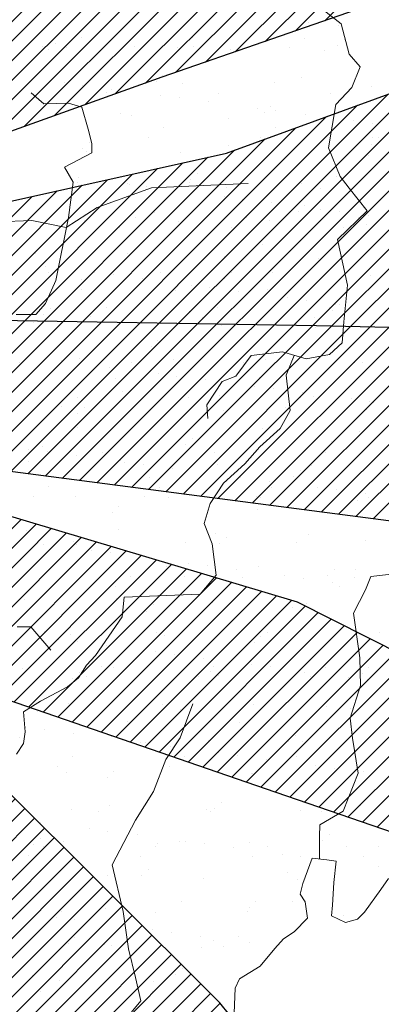
# Model space of a CAD drawing. Units: inches. Extents: x 1986 to 21484, y -1816 to 2016.
# Tile 30 of 85: x 2179.1 to 2183.13, y 1876.39 to 1887.36. Entities that reach past the tile are written whole.
import ezdxf

# ---------------------------------------------------------------- set-up
doc = ezdxf.new("R2010")
doc.units = ezdxf.units.IN
doc.layers.add('L-PLNT', color=84, linetype='Continuous', lineweight=13)
doc.layers.add('vfolhas', color=114, linetype='Continuous', lineweight=5)
for name, color, linetype in [('vfolha', 72, 'Continuous'), ('vfolha2', 110, 'Continuous'), ('vfolhas2', 102, 'Continuous')]:
    doc.layers.add(name, color=color, linetype=linetype)
pattern_1 = [(45, (-2446.5133113, 50.986076), (-0.004419417382, 0.004419417382), [])]

# ---------------------------------------------------------------- blocks, each defined once
blk = doc.blocks.new('arbusto_PB_verde_grande')
at = {"layer": 'vfolha2'}
h = blk.add_hatch(dxfattribs=at)
h.set_pattern_fill('ANSI31', color=256, scale=0.05, style=0)
h.set_pattern_definition(pattern_1)
h.paths.add_polyline_path([(0.02944, 0.35651), (0.00028, 0.09048), (0.02625, -0.03934), (0.047, 0.06233), (0.06189, 0.09731), (0.09372, 0.26573), (0.09955, 0.43473), (0.08789, 0.61313), (0.0645, 0.72266), (0.04988, 0.6851), (0.0236, 0.51294)])
h.paths.add_polyline_path([(0.30106, 0.43789), (0.14225, 0.24871), (0.26685, 0.30022)])
h.paths.add_polyline_path([(0.37995, 0.22817), (0.23697, 0.15193), (0.18428, 0.09364), (0.11122, 0.04358), (0.02625, -0.03934), (0.28061, 0.04667), (0.36829, 0.07798), (0.46756, 0.11239), (0.61068, 0.19376), (0.71585, 0.27823), (0.55813, 0.25948)])
h.paths.add_polyline_path([(0.56101, -0.29441), (0.72752, -0.32573), (0.59024, -0.2412), (0.42962, -0.15982), (0.02625, -0.03934), (0.14922, -0.14107), (0.18838, -0.16604), (0.41501, -0.24435)])
h.paths.add_polyline_path([(-0.27429, -0.44776), (-0.30352, -0.72628), (-0.23923, -0.64175), (-0.15457, -0.45716), (0.02625, -0.03934), (-0.16328, -0.25376)])
h.paths.add_polyline_path([(-0.51963, -0.24744), (-0.67736, -0.32573), (-0.59558, -0.35072), (-0.40574, -0.32882), (-0.21007, -0.20995), (0.02625, -0.03934), (-0.14874, -0.06595), (-0.31518, -0.09101), (-0.41452, -0.15048)])
h.paths.add_polyline_path([(-0.52546, 0.25007), (-0.70947, 0.24698), (-0.51963, 0.1093), (-0.32979, 0.02167), (-0.07567, -0.0128), (-0.04234, -0.02148), (-0.35024, 0.1312)])
at = {"layer": 'vfolhas'}
h = blk.add_hatch(dxfattribs=at)
h.set_pattern_fill('ANSI31', color=256, scale=0.05, style=0)
h.set_pattern_definition(pattern_1)
h.paths.add_polyline_path([(-0.07279, 0.50669), (-0.18085, 0.65063), (-0.2334, 0.67253), (-0.20712, 0.53176), (-0.10785, 0.25007), (0.02625, -0.03934), (0.00028, 0.09048), (0.00816, 0.16241), (-0.04939, 0.29079)])
h.paths.add_polyline_path([(0.09902, 0.41929), (0.09372, 0.26573), (0.07906, 0.18814), (0.15506, 0.36901), (0.26606, 0.5505), (0.28356, 0.63504), (0.2485, 0.68819), (0.25145, 0.63504), (0.20178, 0.54426)])
h.paths.add_polyline_path([(0.12295, 0.24073), (0.047, 0.06233), (0.02625, -0.03934), (0.11122, 0.04358), (0.18428, 0.09364), (0.27478, 0.19376), (0.3215, 0.25323), (0.44129, 0.38467), (0.47634, 0.57866), (0.41789, 0.45347), (0.28939, 0.30954)])
h.paths.add_polyline_path([(0.58145, -0.03779), (0.70707, 0.01536), (0.78591, 0.04667), (0.74796, 0.06549), (0.62818, 0.08423), (0.52595, 0.09048), (0.39745, 0.04358), (0.02625, -0.03934), (0.25728, -0.03154), (0.43834, -0.0347)])
h.paths.add_polyline_path([(0.52022, -0.03647), (0.43834, -0.0347), (0.25728, -0.03154), (0.02625, -0.03934), (0.17964, -0.08515), (0.53768, -0.13167), (0.69541, -0.15357), (0.78591, -0.07852), (0.70413, -0.10042)])
h.paths.add_polyline_path([(0.27189, -0.21929), (0.14922, -0.14107), (0.02625, -0.03934), (0.15794, -0.31007), (0.29522, -0.42585), (0.41789, -0.49157), (0.56396, -0.56669), (0.5114, -0.48532), (0.39456, -0.34139)])
h.paths.add_polyline_path([(-0.05818, -0.47591), (-0.02312, -0.61984), (0.047, -0.80134), (0.08494, -0.59794), (0.07911, -0.4071), (0.03527, -0.25376), (0.02625, -0.03934), (-0.03773, -0.26001)])
h.paths.add_polyline_path([(-0.24218, 0.14054), (-0.11073, 0.06858), (0.02625, -0.03934), (-0.04235, 0.10871), (-0.21007, 0.23757), (-0.36485, 0.33145), (-0.47874, 0.40341), (-0.54303, 0.46288), (-0.49041, 0.33145), (-0.39408, 0.22192)])
at = {"layer": 'vfolha'}
for p, q in [((0.53768, -0.13167), (0.17964, -0.08515)), ((0.39456, -0.34139), (0.27189, -0.21929)), ((0.5114, -0.48532), (0.39456, -0.34139))]:
    blk.add_line(p, q, dxfattribs=at)
at = {"layer": 'vfolha2'}
for p, q in [((0.36829, 0.07798), (0.28061, 0.04667)), ((0.42962, -0.15982), (0.02625, -0.03934)), ((0.59024, -0.2412), (0.42962, -0.15982)), ((0.18838, -0.16604), (0.41501, -0.24435)), ((0.41501, -0.24435), (0.56101, -0.29441))]:
    blk.add_line(p, q, dxfattribs=at)
at = {"layer": 'vfolhas2'}
for p, q in [((0.46756, 0.11239), (0.36829, 0.07798)), ((0.39745, 0.04358), (0.52595, 0.09048)), ((0.02625, -0.03934), (0.39745, 0.04358)), ((0.43834, -0.0347), (0.25728, -0.03154)), ((0.58145, -0.03779), (0.43834, -0.0347))]:
    blk.add_line(p, q, dxfattribs=at)
blk = doc.blocks.new('PLANT-SHRUB')
for p, q in [((2182.269, 1887.643), (2182.682, 1887.317)), ((2182.322, 1887.338), (2182.322, 1887.338)), ((2182.647, 1887.295), (2182.647, 1887.295)), ((2182.682, 1887.317), (2182.772, 1886.981)), ((2182.682, 1887.317), (2182.682, 1887.317)), ((2179.784, 1887.163), (2179.784, 1887.163)), ((2181.029, 1887.161), (2181.029, 1887.161)), ((2182.274, 1887.159), (2182.274, 1887.159)), ((2179.352, 1887.066), (2179.352, 1887.066)), ((2179.492, 1887.099), (2179.492, 1887.099)), ((2179.616, 1887.056), (2179.616, 1887.056)), ((2180.374, 1887.071), (2180.374, 1887.071)), ((2180.861, 1887.054), (2180.861, 1887.054)), ((2181.041, 1887.066), (2181.041, 1887.066)), ((2182.105, 1887.051), (2182.105, 1887.051)), ((2182.641, 1887.08), (2182.641, 1887.08)), ((2182.714, 1887.148), (2182.714, 1887.148)), ((2179.419, 1887.031), (2179.419, 1887.031)), ((2181.453, 1887.032), (2181.453, 1887.032)), ((2182.5, 1887.018), (2182.5, 1887.018)), ((2182.772, 1886.981), (2182.892, 1886.841)), ((2182.892, 1886.841), (2182.802, 1886.61)), ((2182.892, 1886.841), (2182.892, 1886.841)), ((2180.694, 1886.748), (2180.694, 1886.748)), ((2182.243, 1886.716), (2182.243, 1886.716)), ((2179.594, 1886.662), (2179.594, 1886.662)), ((2179.802, 1886.635), (2179.802, 1886.635)), ((2179.867, 1886.67), (2179.867, 1886.67)), ((2180.62, 1886.68), (2180.62, 1886.68)), ((2180.913, 1886.657), (2180.913, 1886.657)), ((2181.935, 1886.662), (2181.935, 1886.662)), ((2182.802, 1886.61), (2182.621, 1886.419)), ((2183.015, 1886.623), (2183.015, 1886.623)), ((2179.227, 1886.548), (2179.368, 1886.425)), ((2180.068, 1886.549), (2180.068, 1886.549)), ((2180.127, 1886.592), (2180.127, 1886.592)), ((2180.67, 1886.52), (2180.67, 1886.52)), ((2180.878, 1886.493), (2180.878, 1886.493)), ((2181.313, 1886.547), (2181.313, 1886.547)), ((2182.558, 1886.544), (2182.558, 1886.544)), ((2179.368, 1886.425), (2179.641, 1886.434)), ((2179.641, 1886.434), (2179.79, 1886.39)), ((2179.79, 1886.39), (2179.86, 1886.144)), ((2181.203, 1886.45), (2181.203, 1886.45)), ((2181.895, 1886.397), (2181.895, 1886.397)), ((2182.621, 1886.419), (2182.54, 1885.937)), ((2180.222, 1886.316), (2180.222, 1886.316)), ((2180.349, 1886.301), (2180.349, 1886.301)), ((2181.746, 1886.379), (2181.746, 1886.379)), ((2181.822, 1886.329), (2181.822, 1886.329)), ((2181.954, 1886.351), (2181.954, 1886.351)), ((2182.279, 1886.309), (2182.279, 1886.309)), ((2181.428, 1886.262), (2181.428, 1886.262)), ((2182.474, 1886.248), (2182.474, 1886.248)), ((2182.822, 1886.237), (2182.822, 1886.237)), ((2183.03, 1886.21), (2183.03, 1886.21)), ((2179.86, 1886.144), (2179.904, 1885.986)), ((2180.538, 1886.053), (2180.538, 1886.053)), ((2180.706, 1886.16), (2180.706, 1886.16)), ((2181.951, 1886.158), (2181.951, 1886.158)), ((2179.875, 1885.997), (2179.875, 1885.997)), ((2179.904, 1885.986), (2179.904, 1885.881)), ((2181.424, 1885.965), (2181.424, 1885.965)), ((2181.782, 1886.05), (2181.782, 1886.05)), ((2183.023, 1885.979), (2183.023, 1885.979)), ((2183.027, 1886.048), (2183.027, 1886.048)), ((2183.097, 1886.046), (2183.097, 1886.046)), ((2179.904, 1885.881), (2179.597, 1885.722)), ((2179.801, 1885.93), (2179.801, 1885.93)), ((2179.842, 1885.9), (2179.842, 1885.9)), ((2180.888, 1885.887), (2180.888, 1885.887)), ((2181.91, 1885.892), (2181.91, 1885.892)), ((2182.54, 1885.937), (2182.671, 1885.616)), ((2182.99, 1885.853), (2182.99, 1885.853)), ((2179.597, 1885.722), (2179.693, 1885.555)), ((2181.076, 1885.646), (2181.076, 1885.646)), ((2182.625, 1885.614), (2182.625, 1885.614)), ((2182.671, 1885.616), (2182.772, 1885.485)), ((2179.693, 1885.555), (2179.641, 1885.16)), ((2179.746, 1885.548), (2179.746, 1885.548)), ((2179.759, 1885.606), (2179.759, 1885.606)), ((2180.301, 1885.534), (2180.301, 1885.534)), ((2180.324, 1885.53), (2180.324, 1885.53)), ((2180.51, 1885.507), (2180.51, 1885.507)), ((2180.568, 1885.489), (2181.646, 1885.537)), ((2180.99, 1885.546), (2180.99, 1885.546)), ((2181.002, 1885.579), (2181.002, 1885.579)), ((2182.235, 1885.544), (2182.235, 1885.544)), ((2179.962, 1885.271), (2180.568, 1885.489)), ((2180.834, 1885.464), (2180.834, 1885.464)), ((2181.403, 1885.492), (2181.403, 1885.492)), ((2182.449, 1885.478), (2182.449, 1885.478)), ((2182.772, 1885.485), (2182.973, 1885.234)), ((2181.377, 1885.392), (2181.377, 1885.392)), ((2181.585, 1885.365), (2181.585, 1885.365)), ((2181.91, 1885.322), (2181.91, 1885.322)), ((2182.278, 1885.296), (2182.278, 1885.296)), ((2179.618, 1885.049), (2179.962, 1885.271)), ((2180.605, 1885.214), (2180.605, 1885.214)), ((2182.204, 1885.228), (2182.204, 1885.228)), ((2182.453, 1885.251), (2182.453, 1885.251)), ((2182.973, 1885.234), (2182.641, 1884.913)), ((2182.661, 1885.223), (2182.661, 1885.223)), ((2182.986, 1885.181), (2182.986, 1885.181)), ((2178.228, 1885.089), (2179.234, 1885.126)), ((2179.234, 1885.126), (2179.618, 1885.049)), ((2179.641, 1885.16), (2179.5, 1884.457)), ((2179.816, 1885.13), (2179.816, 1885.13)), ((2180.384, 1885.159), (2180.384, 1885.159)), ((2180.863, 1885.117), (2180.863, 1885.117)), ((2181.628, 1885.157), (2181.628, 1885.157)), ((2181.885, 1885.122), (2181.885, 1885.122)), ((2182.873, 1885.155), (2182.873, 1885.155)), ((2182.965, 1885.083), (2182.965, 1885.083)), ((2180.215, 1885.052), (2180.215, 1885.052)), ((2181.46, 1885.05), (2181.46, 1885.05)), ((2182.704, 1885.047), (2182.704, 1885.047)), ((2180.257, 1884.896), (2180.257, 1884.896)), ((2181.806, 1884.864), (2181.806, 1884.864)), ((2182.641, 1884.913), (2182.752, 1884.406)), ((2179.276, 1884.755), (2179.276, 1884.755)), ((2180.183, 1884.828), (2180.183, 1884.828)), ((2180.298, 1884.76), (2180.298, 1884.76)), ((2181.378, 1884.721), (2181.378, 1884.721)), ((2182.424, 1884.708), (2182.424, 1884.708)), ((2179.39, 1884.619), (2179.39, 1884.619)), ((2179.423, 1884.547), (2179.423, 1884.547)), ((2179.933, 1884.548), (2179.933, 1884.548)), ((2180.141, 1884.52), (2180.141, 1884.52)), ((2180.668, 1884.545), (2180.668, 1884.545)), ((2181.458, 1884.545), (2181.458, 1884.545)), ((2181.912, 1884.543), (2181.912, 1884.543)), ((2179.5, 1884.457), (2179.386, 1884.202)), ((2179.785, 1884.464), (2179.785, 1884.464)), ((2180.466, 1884.478), (2180.466, 1884.478)), ((2181.009, 1884.406), (2181.009, 1884.406)), ((2181.385, 1884.477), (2181.385, 1884.477)), ((2182.752, 1884.406), (2182.712, 1883.995)), ((2182.752, 1884.406), (2182.752, 1884.406)), ((2183.007, 1884.513), (2183.007, 1884.513)), ((2179.791, 1884.36), (2179.791, 1884.36)), ((2180.837, 1884.347), (2180.837, 1884.347)), ((2181.217, 1884.379), (2181.217, 1884.379)), ((2181.542, 1884.336), (2181.542, 1884.336)), ((2181.86, 1884.352), (2181.86, 1884.352)), ((2182.939, 1884.313), (2182.939, 1884.313)), ((2179.386, 1884.202), (2179.28, 1884.079)), ((2182.085, 1884.265), (2182.085, 1884.265)), ((2182.293, 1884.237), (2182.293, 1884.237)), ((2182.618, 1884.194), (2182.618, 1884.194)), ((2182.66, 1884.194), (2182.66, 1884.194)), ((2179.28, 1884.079), (2179.06, 1884.079)), ((2179.364, 1884.078), (2179.364, 1884.078)), ((2179.438, 1884.145), (2179.438, 1884.145)), ((2180.061, 1884.158), (2180.061, 1884.158)), ((2180.987, 1884.113), (2180.987, 1884.113)), ((2181.305, 1884.156), (2181.305, 1884.156)), ((2182.55, 1884.154), (2182.55, 1884.154)), ((2182.586, 1884.127), (2182.586, 1884.127)), ((2179.251, 1883.985), (2179.251, 1883.985)), ((2179.892, 1884.051), (2179.892, 1884.051)), ((2180.273, 1883.99), (2180.273, 1883.99)), ((2181.137, 1884.049), (2181.137, 1884.049)), ((2182.381, 1884.047), (2182.381, 1884.047)), ((2182.712, 1883.995), (2182.692, 1883.764)), ((2181.353, 1883.951), (2181.353, 1883.951)), ((2182.399, 1883.938), (2182.399, 1883.938)), ((2180.639, 1883.794), (2180.639, 1883.794)), ((2182.188, 1883.762), (2182.188, 1883.762)), ((2182.692, 1883.764), (2182.551, 1883.633)), ((2180.565, 1883.727), (2180.565, 1883.727)), ((2182.029, 1883.663), (2181.677, 1883.623)), ((2182.29, 1883.583), (2182.029, 1883.663)), ((2179.1, 1883.546), (2179.1, 1883.546)), ((2179.564, 1883.561), (2179.564, 1883.561)), ((2179.766, 1883.59), (2179.766, 1883.59)), ((2179.773, 1883.534), (2179.773, 1883.534)), ((2180.345, 1883.544), (2180.345, 1883.544)), ((2180.812, 1883.577), (2180.812, 1883.577)), ((2181.677, 1883.623), (2181.506, 1883.392)), ((2181.589, 1883.542), (2181.589, 1883.542)), ((2181.677, 1883.623), (2181.677, 1883.623)), ((2181.835, 1883.582), (2181.835, 1883.582)), ((2182.159, 1883.623), (2182.068, 1883.402)), ((2182.551, 1883.633), (2182.29, 1883.583)), ((2182.834, 1883.54), (2182.834, 1883.54)), ((2182.914, 1883.543), (2182.914, 1883.543)), ((2180.097, 1883.491), (2180.097, 1883.491)), ((2180.64, 1883.42), (2180.64, 1883.42)), ((2181.841, 1883.443), (2181.841, 1883.443)), ((2180.168, 1883.362), (2180.168, 1883.362)), ((2180.848, 1883.392), (2180.848, 1883.392)), ((2181.173, 1883.35), (2181.173, 1883.35)), ((2181.355, 1883.332), (2181.184, 1883.071)), ((2181.506, 1883.392), (2181.355, 1883.332)), ((2181.355, 1883.332), (2181.355, 1883.332)), ((2181.767, 1883.376), (2181.767, 1883.376)), ((2182.068, 1883.402), (2182.113, 1883.009)), ((2179.226, 1883.215), (2179.226, 1883.215)), ((2180.248, 1883.22), (2180.248, 1883.22)), ((2181.716, 1883.278), (2181.716, 1883.278)), ((2181.924, 1883.251), (2181.924, 1883.251)), ((2182.249, 1883.208), (2182.249, 1883.208)), ((2179.738, 1883.158), (2179.738, 1883.158)), ((2180.983, 1883.155), (2180.983, 1883.155)), ((2181.328, 1883.181), (2181.328, 1883.181)), ((2182.227, 1883.153), (2182.227, 1883.153)), ((2182.374, 1883.168), (2182.374, 1883.168)), ((2182.792, 1883.137), (2182.792, 1883.137)), ((2183, 1883.109), (2183, 1883.109)), ((2183.042, 1883.093), (2183.042, 1883.093)), ((2179.569, 1883.05), (2179.569, 1883.05)), ((2179.82, 1883.044), (2179.82, 1883.044)), ((2180.814, 1883.048), (2180.814, 1883.048)), ((2181.184, 1883.071), (2181.194, 1882.92)), ((2181.369, 1883.011), (2181.369, 1883.011)), ((2182.113, 1883.009), (2182, 1882.806)), ((2182.059, 1883.046), (2182.059, 1883.046)), ((2182.968, 1883.025), (2182.968, 1883.025)), ((2179.746, 1882.976), (2179.746, 1882.976)), ((2179.741, 1882.82), (2179.741, 1882.82)), ((2180.787, 1882.807), (2180.787, 1882.807)), ((2182, 1882.806), (2181.775, 1882.603)), ((2181.81, 1882.811), (2181.81, 1882.811)), ((2182, 1882.806), (2182, 1882.806)), ((2182.889, 1882.773), (2182.889, 1882.773)), ((2181.021, 1882.693), (2181.021, 1882.693)), ((2182.571, 1882.661), (2182.571, 1882.661)), ((2179.196, 1882.575), (2179.196, 1882.575)), ((2179.348, 1882.612), (2179.348, 1882.612)), ((2179.404, 1882.548), (2179.404, 1882.548)), ((2180.022, 1882.543), (2180.022, 1882.543)), ((2180.948, 1882.625), (2180.948, 1882.625)), ((2181.267, 1882.541), (2181.267, 1882.541)), ((2181.775, 1882.603), (2181.606, 1882.412)), ((2179.201, 1882.445), (2179.201, 1882.445)), ((2179.729, 1882.505), (2179.729, 1882.505)), ((2180.223, 1882.45), (2180.223, 1882.45)), ((2180.272, 1882.434), (2180.272, 1882.434)), ((2182.511, 1882.539), (2182.511, 1882.539)), ((2180.48, 1882.406), (2180.48, 1882.406)), ((2180.805, 1882.363), (2180.805, 1882.363)), ((2181.302, 1882.411), (2181.302, 1882.411)), ((2181.606, 1882.412), (2181.369, 1882.198)), ((2182.223, 1882.342), (2182.223, 1882.342)), ((2182.349, 1882.398), (2182.349, 1882.398)), ((2180.55, 1882.261), (2180.55, 1882.261)), ((2181.348, 1882.292), (2181.348, 1882.292)), ((2181.556, 1882.265), (2181.556, 1882.265)), ((2181.881, 1882.222), (2181.881, 1882.222)), ((2182.149, 1882.275), (2182.149, 1882.275)), ((2179.415, 1882.157), (2179.415, 1882.157)), ((2180.66, 1882.155), (2180.66, 1882.155)), ((2181.369, 1882.198), (2181.223, 1881.973)), ((2181.904, 1882.152), (2181.904, 1882.152)), ((2182.423, 1882.15), (2182.423, 1882.15)), ((2182.631, 1882.123), (2182.631, 1882.123)), ((2179.247, 1882.049), (2179.247, 1882.049)), ((2179.716, 1882.05), (2179.716, 1882.05)), ((2180.491, 1882.047), (2180.491, 1882.047)), ((2180.762, 1882.036), (2180.762, 1882.036)), ((2181.736, 1882.045), (2181.736, 1882.045)), ((2181.784, 1882.041), (2181.784, 1882.041)), ((2182.864, 1882.002), (2182.864, 1882.002)), ((2182.956, 1882.08), (2182.956, 1882.08)), ((2182.981, 1882.043), (2182.981, 1882.043)), ((2180.202, 1881.942), (2180.202, 1881.942)), ((2181.223, 1881.973), (2181.155, 1881.748)), ((2181.751, 1881.91), (2181.751, 1881.91)), ((2180.129, 1881.875), (2180.129, 1881.875)), ((2179.175, 1881.675), (2179.175, 1881.675)), ((2180.198, 1881.68), (2180.198, 1881.68)), ((2181.155, 1881.748), (2181.245, 1881.523)), ((2181.277, 1881.641), (2181.277, 1881.641)), ((2181.404, 1881.591), (2181.404, 1881.591)), ((2182.323, 1881.628), (2182.323, 1881.628)), ((2182.953, 1881.559), (2182.953, 1881.559)), ((2179.36, 1881.519), (2179.36, 1881.519)), ((2179.699, 1881.543), (2179.699, 1881.543)), ((2179.731, 1881.51), (2179.731, 1881.51)), ((2179.903, 1881.447), (2179.903, 1881.447)), ((2180.944, 1881.54), (2180.944, 1881.54)), ((2181.245, 1881.523), (2181.29, 1881.174)), ((2181.33, 1881.524), (2181.33, 1881.524)), ((2182.188, 1881.538), (2182.188, 1881.538)), ((2180.111, 1881.42), (2180.111, 1881.42)), ((2180.436, 1881.377), (2180.436, 1881.377)), ((2179.691, 1881.28), (2179.691, 1881.28)), ((2180.737, 1881.266), (2180.737, 1881.266)), ((2180.979, 1881.306), (2180.979, 1881.306)), ((2181.187, 1881.278), (2181.187, 1881.278)), ((2181.512, 1881.235), (2181.512, 1881.235)), ((2181.759, 1881.271), (2181.759, 1881.271)), ((2182.605, 1881.241), (2182.605, 1881.241)), ((2182.839, 1881.232), (2182.839, 1881.232)), ((2179.309, 1881.124), (2179.309, 1881.124)), ((2179.383, 1881.192), (2179.383, 1881.192)), ((2180.337, 1881.154), (2180.337, 1881.154)), ((2180.932, 1881.159), (2180.932, 1881.159)), ((2181.29, 1881.174), (2181.11, 1880.96)), ((2181.582, 1881.151), (2181.582, 1881.151)), ((2182.055, 1881.164), (2182.055, 1881.164)), ((2182.263, 1881.137), (2182.263, 1881.137)), ((2182.532, 1881.173), (2182.532, 1881.173)), ((2182.826, 1881.149), (2182.826, 1881.149)), ((2182.952, 1881.008), (2183.014, 1881.159)), ((2183.014, 1881.159), (2183.422, 1881.204)), ((2183.014, 1881.159), (2183.014, 1881.159)), ((2180.169, 1881.046), (2180.169, 1881.046)), ((2181.413, 1881.044), (2181.413, 1881.044)), ((2182.588, 1881.094), (2182.588, 1881.094)), ((2182.658, 1881.042), (2182.658, 1881.042)), ((2182.819, 1880.751), (2182.952, 1881.008)), ((2179.15, 1880.905), (2179.15, 1880.905)), ((2180.173, 1880.91), (2180.173, 1880.91)), ((2180.262, 1880.928), (2180.242, 1880.708)), ((2181.11, 1880.96), (2180.262, 1880.928)), ((2181.11, 1880.96), (2181.11, 1880.96)), ((2180.585, 1880.841), (2180.585, 1880.841)), ((2181.252, 1880.871), (2181.252, 1880.871)), ((2182.134, 1880.809), (2182.134, 1880.809)), ((2182.298, 1880.858), (2182.298, 1880.858)), ((2180.242, 1880.708), (2179.942, 1880.278)), ((2180.511, 1880.773), (2180.511, 1880.773)), ((2182.889, 1880.253), (2182.819, 1880.751)), ((2179.071, 1880.597), (2179.221, 1880.597)), ((2179.221, 1880.597), (2179.446, 1880.335)), ((2179.376, 1880.542), (2179.376, 1880.542)), ((2179.535, 1880.461), (2179.535, 1880.461)), ((2179.665, 1880.51), (2179.665, 1880.51)), ((2180.621, 1880.539), (2180.621, 1880.539)), ((2180.712, 1880.496), (2180.712, 1880.496)), ((2181.734, 1880.501), (2181.734, 1880.501)), ((2181.786, 1880.49), (2181.786, 1880.49)), ((2181.866, 1880.537), (2181.866, 1880.537)), ((2182.813, 1880.462), (2182.813, 1880.462)), ((2183.11, 1880.535), (2183.11, 1880.535)), ((2179.743, 1880.434), (2179.743, 1880.434)), ((2180.068, 1880.391), (2180.068, 1880.391)), ((2180.113, 1880.409), (2180.113, 1880.409)), ((2181.712, 1880.422), (2181.712, 1880.422)), ((2179.942, 1880.278), (2179.842, 1880.168)), ((2180.611, 1880.319), (2180.611, 1880.319)), ((2180.819, 1880.292), (2180.819, 1880.292)), ((2181.144, 1880.249), (2181.144, 1880.249)), ((2182.898, 1879.943), (2182.889, 1880.253)), ((2179.125, 1880.135), (2179.125, 1880.135)), ((2179.842, 1880.168), (2179.752, 1880.028)), ((2180.014, 1880.153), (2180.014, 1880.153)), ((2180.147, 1880.14), (2180.147, 1880.14)), ((2181.259, 1880.151), (2181.259, 1880.151)), ((2181.686, 1880.178), (2181.686, 1880.178)), ((2181.895, 1880.15), (2181.895, 1880.15)), ((2182.504, 1880.148), (2182.504, 1880.148)), ((2182.987, 1880.139), (2182.987, 1880.139)), ((2179.752, 1880.028), (2179.632, 1879.928)), ((2179.692, 1880.023), (2179.692, 1880.023)), ((2179.765, 1880.09), (2179.765, 1880.09)), ((2179.846, 1880.046), (2179.846, 1880.046)), ((2181.09, 1880.043), (2181.09, 1880.043)), ((2181.227, 1880.101), (2181.227, 1880.101)), ((2181.315, 1880.058), (2181.315, 1880.058)), ((2182.219, 1880.108), (2182.219, 1880.108)), ((2182.273, 1880.088), (2182.273, 1880.088)), ((2182.335, 1880.041), (2182.335, 1880.041)), ((2182.762, 1880.036), (2182.762, 1880.036)), ((2182.914, 1880.072), (2182.914, 1880.072)), ((2179.632, 1879.928), (2179.331, 1879.768)), ((2179.632, 1879.928), (2179.632, 1879.928)), ((2182.782, 1879.579), (2182.898, 1879.943)), ((2182.97, 1880.009), (2182.97, 1880.009)), ((2179.331, 1879.768), (2179.141, 1879.648)), ((2179.64, 1879.739), (2179.64, 1879.739)), ((2180.686, 1879.726), (2180.686, 1879.726)), ((2181.028, 1879.737), (2180.888, 1879.358)), ((2180.967, 1879.739), (2180.967, 1879.739)), ((2181.709, 1879.731), (2181.709, 1879.731)), ((2182.516, 1879.707), (2182.516, 1879.707)), ((2182.788, 1879.692), (2182.788, 1879.692)), ((2179.141, 1879.648), (2179.161, 1879.428)), ((2179.294, 1879.658), (2179.294, 1879.658)), ((2180.893, 1879.672), (2180.893, 1879.672)), ((2182.809, 1879.357), (2182.782, 1879.579)), ((2179.166, 1879.475), (2179.166, 1879.475)), ((2180.298, 1879.539), (2180.298, 1879.539)), ((2181.543, 1879.536), (2181.543, 1879.536)), ((2182.787, 1879.534), (2182.787, 1879.534)), ((2179.1, 1879.365), (2179.1, 1879.365)), ((2179.161, 1879.428), (2179.141, 1879.298)), ((2179.374, 1879.447), (2179.374, 1879.447)), ((2179.699, 1879.404), (2179.699, 1879.404)), ((2180.122, 1879.37), (2180.122, 1879.37)), ((2180.888, 1879.358), (2180.729, 1879.119)), ((2182.168, 1879.389), (2182.168, 1879.389)), ((2182.871, 1878.967), (2182.809, 1879.357)), ((2179.141, 1879.298), (2179.061, 1879.179)), ((2180.242, 1879.333), (2180.242, 1879.333)), ((2180.45, 1879.306), (2180.45, 1879.306)), ((2180.495, 1879.307), (2180.495, 1879.307)), ((2180.775, 1879.263), (2180.775, 1879.263)), ((2181.202, 1879.331), (2181.202, 1879.331)), ((2182.095, 1879.321), (2182.095, 1879.321)), ((2182.248, 1879.317), (2182.248, 1879.317)), ((2179.691, 1879.152), (2179.691, 1879.152)), ((2180.936, 1879.15), (2180.936, 1879.15)), ((2181.318, 1879.191), (2181.318, 1879.191)), ((2181.526, 1879.164), (2181.526, 1879.164)), ((2182.181, 1879.148), (2182.181, 1879.148)), ((2179.523, 1879.045), (2179.523, 1879.045)), ((2180.729, 1879.119), (2180.589, 1878.76)), ((2180.768, 1879.042), (2180.768, 1879.042)), ((2181.851, 1879.121), (2181.851, 1879.121)), ((2182.012, 1879.04), (2182.012, 1879.04)), ((2182.394, 1879.05), (2182.394, 1879.05)), ((2179.615, 1878.969), (2179.615, 1878.969)), ((2180.074, 1878.921), (2180.074, 1878.921)), ((2180.148, 1878.989), (2180.148, 1878.989)), ((2180.661, 1878.956), (2180.661, 1878.956)), ((2181.684, 1878.961), (2181.684, 1878.961)), ((2181.697, 1878.957), (2181.697, 1878.957)), ((2182.602, 1879.022), (2182.602, 1879.022)), ((2182.702, 1878.542), (2182.871, 1878.967)), ((2182.763, 1878.922), (2182.763, 1878.922)), ((2182.927, 1878.98), (2182.927, 1878.98)), ((2180.589, 1878.76), (2180.389, 1878.441)), ((2180.097, 1878.6), (2180.097, 1878.6)), ((2181.349, 1878.638), (2181.349, 1878.638)), ((2182.898, 1878.606), (2182.898, 1878.606)), ((2179.676, 1878.557), (2179.676, 1878.557)), ((2179.975, 1878.538), (2179.975, 1878.538)), ((2181.176, 1878.561), (2181.176, 1878.561)), ((2181.22, 1878.536), (2181.22, 1878.536)), ((2181.275, 1878.57), (2181.275, 1878.57)), ((2182.223, 1878.547), (2182.223, 1878.547)), ((2182.445, 1878.391), (2182.702, 1878.542)), ((2182.465, 1878.533), (2182.465, 1878.533)), ((2179.331, 1878.418), (2179.331, 1878.418)), ((2180.389, 1878.441), (2180.13, 1877.943)), ((2180.389, 1878.441), (2180.389, 1878.441)), ((2182.44, 1878.258), (2182.445, 1878.391)), ((2179.874, 1878.347), (2179.874, 1878.347)), ((2180.082, 1878.319), (2180.082, 1878.319)), ((2180.407, 1878.277), (2180.407, 1878.277)), ((2182.551, 1878.287), (2182.551, 1878.287)), ((2179.255, 1878.171), (2179.255, 1878.171)), ((2179.328, 1878.238), (2179.328, 1878.238)), ((2179.369, 1878.151), (2179.369, 1878.151)), ((2179.59, 1878.199), (2179.59, 1878.199)), ((2180.613, 1878.149), (2180.613, 1878.149)), ((2180.636, 1878.186), (2180.636, 1878.186)), ((2180.878, 1878.206), (2180.878, 1878.206)), ((2180.949, 1878.205), (2180.949, 1878.205)), ((2181.158, 1878.178), (2181.158, 1878.178)), ((2181.658, 1878.191), (2181.658, 1878.191)), ((2182.44, 1878.008), (2182.44, 1878.258)), ((2182.477, 1878.22), (2182.477, 1878.22)), ((2182.738, 1878.152), (2182.738, 1878.152)), ((2179.2, 1878.044), (2179.2, 1878.044)), ((2180.445, 1878.042), (2180.445, 1878.042)), ((2181.482, 1878.135), (2181.482, 1878.135)), ((2181.689, 1878.039), (2181.689, 1878.039)), ((2181.858, 1878.147), (2181.858, 1878.147)), ((2182.025, 1878.063), (2182.025, 1878.063)), ((2183.103, 1878.144), (2183.103, 1878.144)), ((2180.13, 1877.943), (2180.25, 1877.424)), ((2182.233, 1878.036), (2182.233, 1878.036)), ((2182.359, 1878.019), (2182.255, 1877.734)), ((2182.359, 1878.019), (2182.359, 1878.019)), ((2182.521, 1877.998), (2182.359, 1878.019)), ((2182.625, 1877.986), (2182.521, 1877.998)), ((2182.558, 1877.993), (2182.558, 1877.993)), ((2182.599, 1877.747), (2182.625, 1877.986)), ((2182.934, 1878.037), (2182.934, 1878.037)), ((2180.072, 1877.829), (2180.072, 1877.829)), ((2180.456, 1877.82), (2180.456, 1877.82)), ((2180.53, 1877.887), (2180.53, 1877.887)), ((2182.079, 1877.855), (2182.079, 1877.855)), ((2183.101, 1877.922), (2183.101, 1877.922)), ((2181.151, 1877.791), (2181.151, 1877.791)), ((2182.197, 1877.777), (2182.197, 1877.777)), ((2182.255, 1877.734), (2182.223, 1877.617)), ((2182.586, 1877.494), (2182.599, 1877.747)), ((2182.599, 1877.747), (2182.599, 1877.747)), ((2183.209, 1877.792), (2183.124, 1877.669)), ((2182.223, 1877.617), (2182.281, 1877.533)), ((2183.124, 1877.669), (2182.943, 1877.416)), ((2179.653, 1877.537), (2179.653, 1877.537)), ((2180.897, 1877.535), (2180.897, 1877.535)), ((2181.731, 1877.537), (2181.731, 1877.537)), ((2182.142, 1877.532), (2182.142, 1877.532)), ((2182.281, 1877.533), (2182.307, 1877.351)), ((2182.573, 1877.377), (2182.586, 1877.494)), ((2182.586, 1877.494), (2182.586, 1877.494)), ((2179.565, 1877.429), (2179.565, 1877.429)), ((2180.058, 1877.455), (2180.058, 1877.455)), ((2180.25, 1877.424), (2180.31, 1877.006)), ((2180.611, 1877.416), (2180.611, 1877.416)), ((2181.633, 1877.421), (2181.633, 1877.421)), ((2181.658, 1877.469), (2181.658, 1877.469)), ((2182.713, 1877.382), (2182.713, 1877.382)), ((2182.943, 1877.416), (2182.865, 1877.338)), ((2179.505, 1877.36), (2179.505, 1877.36)), ((2179.713, 1877.333), (2179.713, 1877.333)), ((2180.038, 1877.29), (2180.038, 1877.29)), ((2182.307, 1877.351), (2182.158, 1877.196)), ((2182.573, 1877.377), (2182.573, 1877.377)), ((2182.729, 1877.3), (2182.573, 1877.377)), ((2182.865, 1877.338), (2182.729, 1877.3)), ((2180.581, 1877.219), (2180.581, 1877.219)), ((2180.789, 1877.191), (2180.789, 1877.191)), ((2182.158, 1877.196), (2182.04, 1877.12)), ((2182.158, 1877.196), (2182.158, 1877.196)), ((2179.637, 1877.069), (2179.637, 1877.069)), ((2179.711, 1877.137), (2179.711, 1877.137)), ((2180.047, 1877.059), (2180.047, 1877.059)), ((2180.291, 1877.148), (2180.291, 1877.148)), ((2181.114, 1877.149), (2181.114, 1877.149)), ((2181.26, 1877.105), (2181.26, 1877.105)), ((2181.535, 1877.146), (2181.535, 1877.146)), ((2181.657, 1877.077), (2181.657, 1877.077)), ((2182.04, 1877.12), (2181.942, 1877.01)), ((2180.122, 1877.041), (2180.122, 1877.041)), ((2180.31, 1877.006), (2180.389, 1876.687)), ((2181.126, 1877.02), (2181.126, 1877.02)), ((2181.367, 1877.039), (2181.367, 1877.039)), ((2181.942, 1877.01), (2181.78, 1876.816)), ((2180.912, 1876.786), (2180.912, 1876.786)), ((2181.78, 1876.816), (2181.547, 1876.673)), ((2179.239, 1876.705), (2179.239, 1876.705)), ((2179.54, 1876.659), (2179.54, 1876.659)), ((2180.389, 1876.687), (2180.449, 1876.428)), ((2180.586, 1876.646), (2180.586, 1876.646)), ((2180.839, 1876.718), (2180.839, 1876.718)), ((2181.547, 1876.673), (2181.501, 1876.57)), ((2179.33, 1876.536), (2179.33, 1876.536)), ((2180.574, 1876.534), (2180.574, 1876.534)), ((2181.501, 1876.57), (2181.488, 1876.291)), ((2180.449, 1876.428), (2180.25, 1876.189)), ((2180.449, 1876.428), (2180.449, 1876.428))]:
    blk.add_line(p, q)

msp = doc.modelspace()

# ---------------------------------------------------------------- block references
at = {"layer": 'L-PLNT'}
msp.add_blockref('PLANT-SHRUB', (0, 0), dxfattribs=at)
at = {"layer": 'L-PLNT', "xscale": 24.60366729364114, "yscale": 24.60366729364114, "zscale": 24.60366729364114}
msp.add_blockref('arbusto_PB_verde_grande', (2171.623, 1884.805), dxfattribs=at)

doc.saveas('drawing.dxf')
